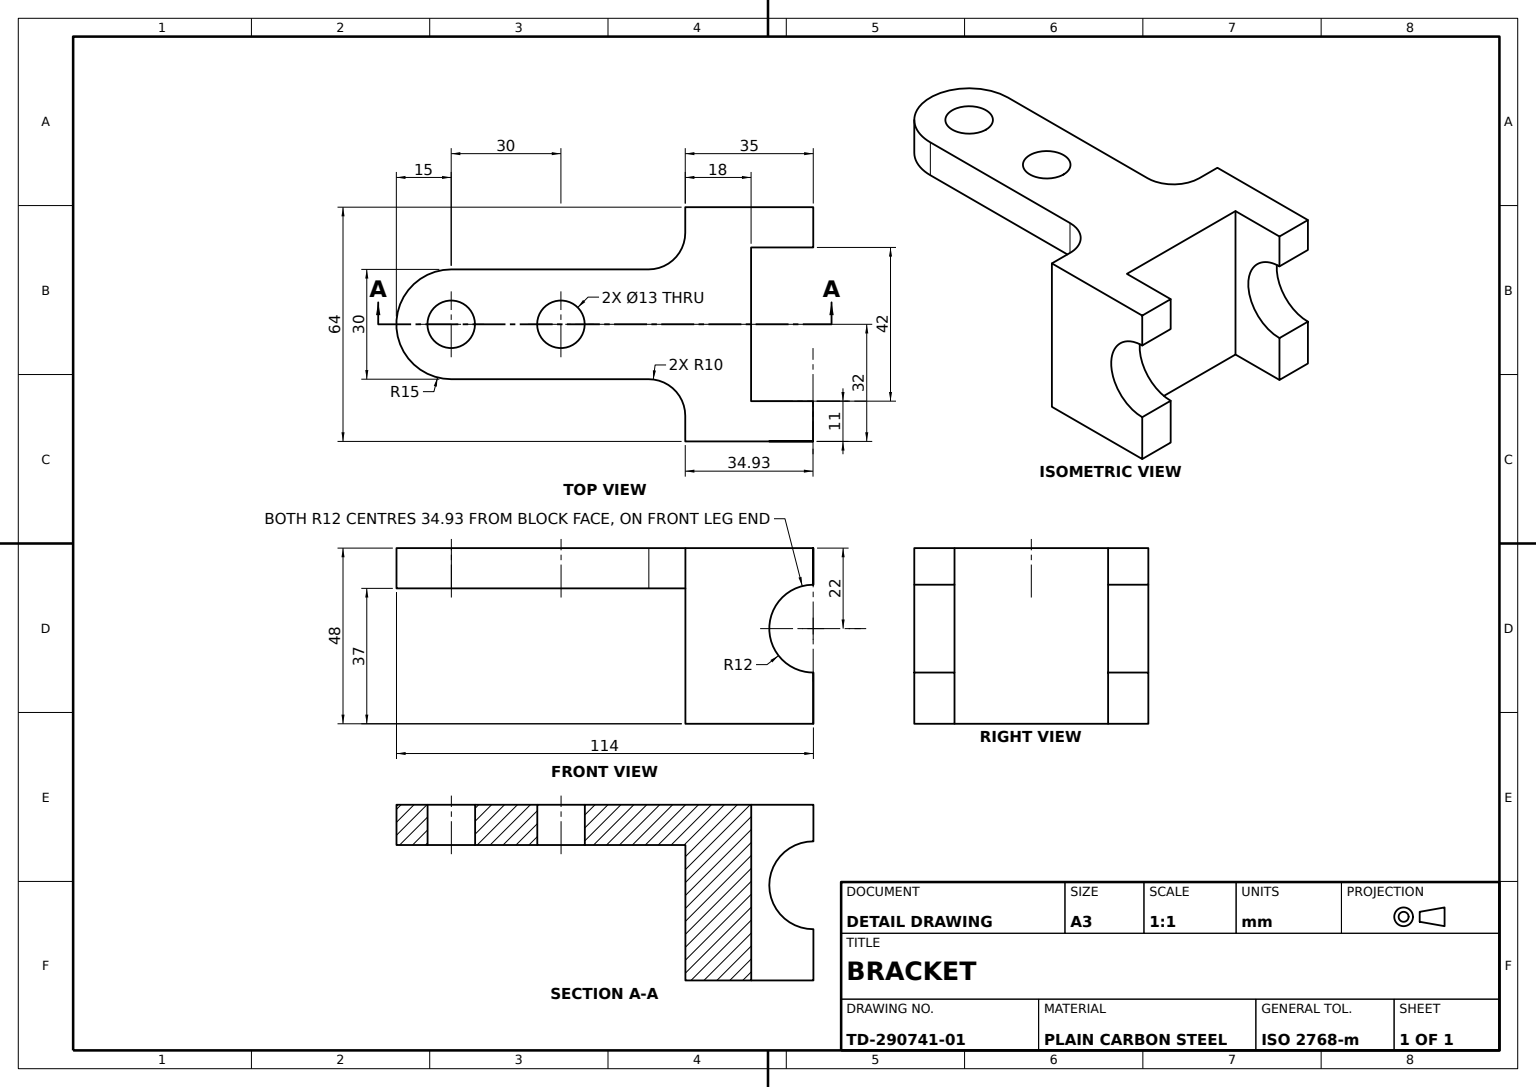
from build123d import *

# Parameters (mm, degrees)
PLATE_PROFILE_SKETCH_R    = 6.5
MOUNTING_PLATE_11MM_DEPTH = 11
SUPPORT_BLOCK_37MM_DEPTH  = 37
FILLET_R10_R              = 10
ARM_HOLE_DEPTH            = 124.555655476
ARM_HOLE_DEPTH_BACK       = 124.555655476
ARM_HOLE_SKETCH_R         = 12


with BuildPart() as part:
    # Plate Profile Sketch → Mounting Plate 11mm (new body)
    with BuildSketch(Plane(origin=(0, 0, 0), x_dir=(1, 0, 0), z_dir=(0, 1, 0))):
        with BuildLine():
            Line((-15, 0), (-15, 64))
            Line((-15, 64), (-32, 64))
            Line((-32, 64), (-32, 99))
            Line((-32, 99), (-21, 99))
            Line((-21, 99), (-21, 82))
            Line((-21, 82), (21, 82))
            Line((21, 82), (21, 98.934064449))
            Line((21, 98.934064449), (32, 98.934064449))
            Line((32, 98.934064449), (32, 64))
            Line((32, 64), (15, 64))
            Line((15, 64), (15, 0))
            ThreePointArc((15, 0), (0, -15), (-15, 0))
        make_face()
        with Locations(Location((0, 0, 0), (0, 0, 270))):
            Circle(PLATE_PROFILE_SKETCH_R, mode=Mode.SUBTRACT)
        with Locations(Location((0, 30, 0), (0, 0, 270))):
            Circle(PLATE_PROFILE_SKETCH_R, mode=Mode.SUBTRACT)
    extrude(amount=MOUNTING_PLATE_11MM_DEPTH)

    # Support Block Sketch → Support Block 37mm (add)
    with BuildSketch(Plane.XZ):
        Polygon((-32, -64), (32, -64), (32, -98.934064449), (21, -98.934064449), (21, -82), (-21, -82), (-21, -99), (-32, -99), align=None)
    extrude(amount=SUPPORT_BLOCK_37MM_DEPTH)

    # Fillet R10
    fillet_r10_edges = [part.edges().sort_by_distance(p)[0] for p in [
        (-15, 5.5, -64),
        (15, 5.5, -64),
    ]]
    fillet(fillet_r10_edges, radius=FILLET_R10_R)

    # Arm Hole Sketch → Arm Hole (cut, two sides: drawn at the far end of the back side and taken through both)
    with BuildSketch(Plane(origin=(32, 0, 0), x_dir=(0, 0, -1), z_dir=(1, 0, 0)).offset(-ARM_HOLE_DEPTH_BACK)):
        with Locations((98.934064449, -11)):
            Circle(ARM_HOLE_SKETCH_R)
    extrude(amount=ARM_HOLE_DEPTH + ARM_HOLE_DEPTH_BACK, mode=Mode.SUBTRACT)


solid = part.part
